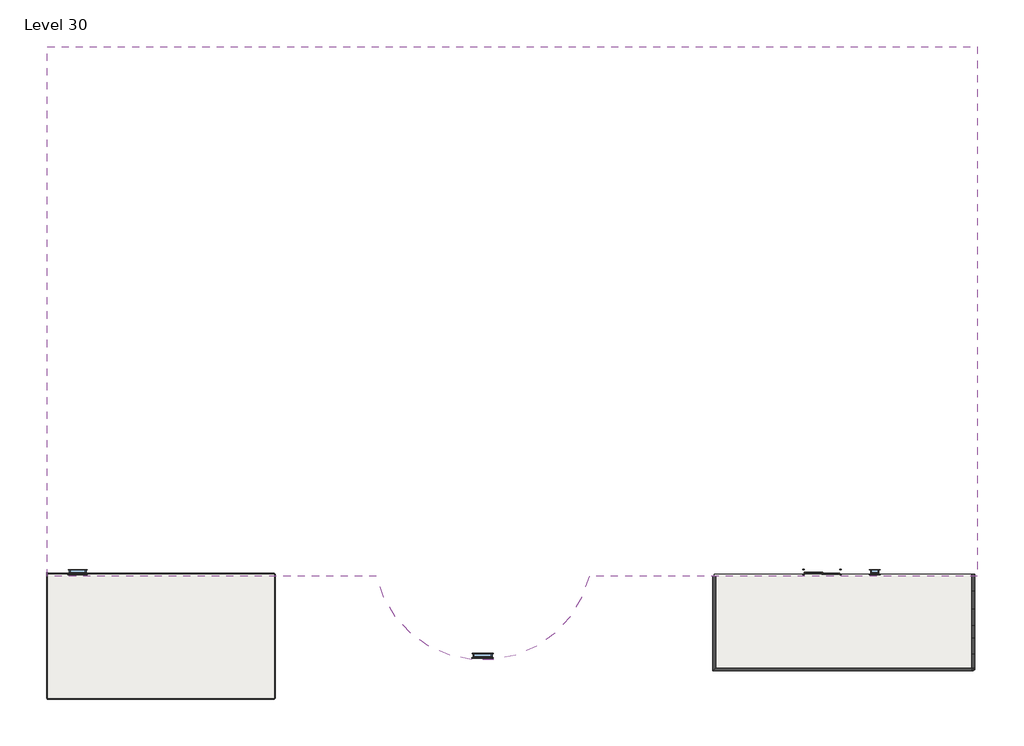
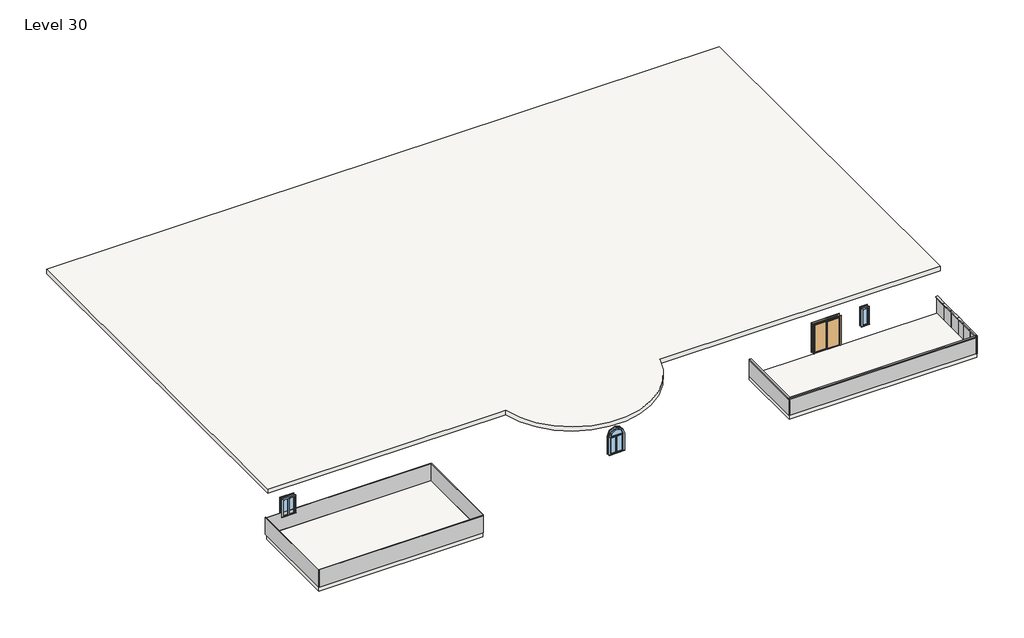
# One storey: 12 plates, 10 members, 3 slabs, 3 windows, 1 door.
"""IFC4 building model written with IfcOpenShell, lengths in millimetres."""

from ifc_helpers import new_model, si_unit, point, frame, frame_2d, origin, place, context, project, spatial, polyline, circle_curve, trimmed, segment, composite_curve, outline, extrude, transform, mapped, element, save
from components import door_076b30e0, member_75074519, member_9ef15e39, member_47bfaf8a, member_aa870034, member_b955a9e9, member_f377c62d, member_60525e8a, system_panel_glazed_689d74eb, system_panel_glazed_59c8d2f2, system_panel_glazed_7b5ce646, system_panel_glazed_f269d4c8, system_panel_glazed_7af1c9c3, system_panel_glazed_dc8eac37, system_panel_glazed_ce931456, system_panel_glazed_5fdeb3e7, system_panel_glazed_fe04ab03, window_cf4adaea, window_a765b88f, window_bb17773d

model = new_model("IFC4")

# Units and contexts
model_context = context("Model", 3, world=origin())
ifc_project = project(units=[si_unit("LENGTHUNIT", "METRE", prefix="MILLI")], contexts=[model_context])

# Site, building, storey
site = spatial("IfcSite", under=ifc_project)
building = spatial("IfcBuilding", under=site)
storey = spatial("IfcBuildingStorey", under=building, Name="Level 30", Elevation=49987.2)

# Door
placement = place(None, origin())
door_shape = door_076b30e0(model_context)
element("IfcDoor", 1, ObjectType="Door-Double-Sliding : 68\" x 80\"", at=placement, inside=storey, context=model_context, shape_type="MappedRepresentation", body=[
    mapped(door_shape, transform((17920.614721, -12227.7237084, 49987.2), x_axis=(-1.0, 0.0, 0.0), y_axis=(0.0, -1.0, 0.0), z_axis=(0.0, 0.0, 1.0))),
])

# Members
member_shape = member_75074519(model_context)
element("IfcMember", 2, ObjectType="Rectangular Mullion : 2.5\" x 5\" rectangular", at=placement, inside=storey, context=model_context, shape_type="MappedRepresentation", body=[
    mapped(member_shape, transform((25286.614721, -17112.9563074, 51206.4), x_axis=(1.0, 0.0, 0.0), y_axis=(0.0, 1.0, 0.0), z_axis=(0.0, 0.0, 1.0))),
])
member_2_shape = member_9ef15e39(model_context)
element("IfcMember", 3, ObjectType="Rectangular Mullion : 2.5\" x 5\" rectangular", at=placement, inside=storey, context=model_context, shape_type="MappedRepresentation", body=[
    mapped(member_2_shape, transform((25286.614721, -13297.3345747, 51206.4), x_axis=(0.0, 0.0, 1.0), y_axis=(-1.0, 0.0, 0.0), z_axis=(0.0, -1.0, 0.0))),
])
element("IfcMember", 4, ObjectType="Rectangular Mullion : 2.5\" x 5\" rectangular", at=placement, inside=storey, context=model_context, shape_type="MappedRepresentation", body=[
    mapped(member_2_shape, transform((25286.614721, -14138.345441, 51206.4), x_axis=(0.0, 0.0, 1.0), y_axis=(-1.0, 0.0, 0.0), z_axis=(0.0, -1.0, 0.0))),
])
element("IfcMember", 5, ObjectType="Rectangular Mullion : 2.5\" x 5\" rectangular", at=placement, inside=storey, context=model_context, shape_type="MappedRepresentation", body=[
    mapped(member_2_shape, transform((25286.614721, -14979.3563074, 51206.4), x_axis=(0.0, 0.0, 1.0), y_axis=(-1.0, 0.0, 0.0), z_axis=(0.0, -1.0, 0.0))),
])
member_3_shape = member_47bfaf8a(model_context)
element("IfcMember", 6, ObjectType="Rectangular Mullion : 2.5\" x 5\" rectangular", at=placement, inside=storey, context=model_context, shape_type="MappedRepresentation", body=[
    mapped(member_3_shape, transform((25286.614721, -15588.9563074, 51206.4), x_axis=(0.0, 0.0, 1.0), y_axis=(-1.0, 0.0, 0.0), z_axis=(0.0, -1.0, 0.0))),
])
member_4_shape = member_aa870034(model_context)
element("IfcMember", 7, ObjectType="Rectangular Mullion : 2.5\" x 5\" rectangular", at=placement, inside=storey, context=model_context, shape_type="MappedRepresentation", body=[
    mapped(member_4_shape, transform((25286.614721, -16350.9563074, 51206.4), x_axis=(0.0, 0.0, 1.0), y_axis=(-1.0, 0.0, 0.0), z_axis=(0.0, -1.0, 0.0))),
])
member_5_shape = member_b955a9e9(model_context)
element("IfcMember", 8, ObjectType="Rectangular Mullion : 2.5\" x 5\" rectangular", at=placement, inside=storey, context=model_context, shape_type="MappedRepresentation", body=[
    mapped(member_5_shape, transform((25286.614721, -17049.4563074, 51206.4), x_axis=(0.0, 0.0, 1.0), y_axis=(-1.0, 0.0, 0.0), z_axis=(0.0, -1.0, 0.0))),
])
element("IfcMember", 9, ObjectType="Rectangular Mullion : 2.5\" x 5\" rectangular", at=placement, inside=storey, context=model_context, shape_type="MappedRepresentation", body=[
    mapped(member_shape, transform((25286.614721, -17112.9563074, 49987.2), x_axis=(0.0, -1.0, 0.0), y_axis=(-1.0, 0.0, 0.0), z_axis=(0.0, 0.0, -1.0))),
])
member_6_shape = member_f377c62d(model_context)
element("IfcMember", 10, ObjectType="Rectangular Mullion : 2.5\" x 5\" rectangular", at=placement, inside=storey, context=model_context, shape_type="MappedRepresentation", body=[
    mapped(member_6_shape, transform((12667.5594464, -12557.9237084, 51206.4), x_axis=(0.0, 0.0, 1.0), y_axis=(1.0, 0.0, 0.0), z_axis=(0.0, 1.0, 0.0))),
])
member_7_shape = member_60525e8a(model_context)
element("IfcMember", 11, ObjectType="Rectangular Mullion : 2.5\" x 5\" rectangular", at=placement, inside=storey, context=model_context, shape_type="MappedRepresentation", body=[
    mapped(member_7_shape, transform((12667.5594464, -17112.9563074, 51206.4), x_axis=(0.0, 0.0, 1.0), y_axis=(0.0, 1.0, 0.0), z_axis=(-1.0, 0.0, 0.0))),
])

# Plates
system_panel_glazed_shape = system_panel_glazed_689d74eb(model_context)
element("IfcPlate", 12, ObjectType="System Panel : Glazed", at=placement, inside=storey, context=model_context, shape_type="MappedRepresentation", body=[
    mapped(system_panel_glazed_shape, transform((18945.3370837, -17112.9563074, 49987.2), x_axis=(-1.0, 0.0, 0.0), y_axis=(0.0, -1.0, 0.0), z_axis=(0.0, 0.0, 1.0))),
])
system_panel_glazed_2_shape = system_panel_glazed_59c8d2f2(model_context)
element("IfcPlate", 13, ObjectType="System Panel : Glazed", at=placement, inside=storey, context=model_context, shape_type="MappedRepresentation", body=[
    mapped(system_panel_glazed_2_shape, transform((25286.614721, -12876.8291415, 49987.2), x_axis=(0.0, -1.0, 0.0), y_axis=(1.0, 0.0, 0.0), z_axis=(0.0, 0.0, 1.0))),
])
element("IfcPlate", 14, ObjectType="System Panel : Glazed", at=placement, inside=storey, context=model_context, shape_type="MappedRepresentation", body=[
    mapped(system_panel_glazed_2_shape, transform((25286.614721, -14558.8508742, 49987.2), x_axis=(0.0, -1.0, 0.0), y_axis=(1.0, 0.0, 0.0), z_axis=(0.0, 0.0, 1.0))),
])
element("IfcPlate", 15, ObjectType="System Panel : Glazed", at=placement, inside=storey, context=model_context, shape_type="MappedRepresentation", body=[
    mapped(system_panel_glazed_2_shape, transform((25286.614721, -13717.8400079, 49987.2), x_axis=(0.0, -1.0, 0.0), y_axis=(1.0, 0.0, 0.0), z_axis=(0.0, 0.0, 1.0))),
])
system_panel_glazed_3_shape = system_panel_glazed_7b5ce646(model_context)
element("IfcPlate", 16, ObjectType="System Panel : Glazed", at=placement, inside=storey, context=model_context, shape_type="MappedRepresentation", body=[
    mapped(system_panel_glazed_3_shape, transform((25286.614721, -16700.2063074, 49987.2), x_axis=(0.0, -1.0, 0.0), y_axis=(1.0, 0.0, 0.0), z_axis=(0.0, 0.0, 1.0))),
])
system_panel_glazed_4_shape = system_panel_glazed_f269d4c8(model_context)
element("IfcPlate", 17, ObjectType="System Panel : Glazed", at=placement, inside=storey, context=model_context, shape_type="MappedRepresentation", body=[
    mapped(system_panel_glazed_4_shape, transform((25286.614721, -15969.9563074, 49987.2), x_axis=(0.0, -1.0, 0.0), y_axis=(1.0, 0.0, 0.0), z_axis=(0.0, 0.0, 1.0))),
])
system_panel_glazed_5_shape = system_panel_glazed_7af1c9c3(model_context)
element("IfcPlate", 18, ObjectType="System Panel : Glazed", at=placement, inside=storey, context=model_context, shape_type="MappedRepresentation", body=[
    mapped(system_panel_glazed_5_shape, transform((25286.614721, -15284.1563074, 49987.2), x_axis=(0.0, -1.0, 0.0), y_axis=(1.0, 0.0, 0.0), z_axis=(0.0, 0.0, 1.0))),
])
system_panel_glazed_6_shape = system_panel_glazed_dc8eac37(model_context)
element("IfcPlate", 19, ObjectType="System Panel : Glazed", at=placement, inside=storey, context=model_context, shape_type="MappedRepresentation", body=[
    mapped(system_panel_glazed_6_shape, transform((12667.5594464, -14835.4400079, 49987.2), x_axis=(0.0, 1.0, 0.0), y_axis=(-1.0, 0.0, 0.0), z_axis=(0.0, 0.0, 1.0))),
])
system_panel_glazed_7_shape = system_panel_glazed_ce931456(model_context)
element("IfcPlate", 20, ObjectType="System Panel : Glazed", at=placement, inside=storey, context=model_context, shape_type="MappedRepresentation", body=[
    mapped(system_panel_glazed_7_shape, transform((-8774.785279, -15482.0987084, 49987.2), x_axis=(0.0, -1.0, 0.0), y_axis=(1.0, 0.0, 0.0), z_axis=(0.0, 0.0, 1.0))),
])
system_panel_glazed_8_shape = system_panel_glazed_5fdeb3e7(model_context)
element("IfcPlate", 21, ObjectType="System Panel : Glazed", at=placement, inside=storey, context=model_context, shape_type="MappedRepresentation", body=[
    mapped(system_panel_glazed_8_shape, transform((-14299.285279, -12456.3237084, 49987.2), x_axis=(1.0, 0.0, 0.0), y_axis=(0.0, 1.0, 0.0), z_axis=(0.0, 0.0, 1.0))),
])
element("IfcPlate", 22, ObjectType="System Panel : Glazed", at=placement, inside=storey, context=model_context, shape_type="MappedRepresentation", body=[
    mapped(system_panel_glazed_8_shape, transform((-14299.285279, -18507.8737084, 49987.2), x_axis=(-1.0, 0.0, 0.0), y_axis=(0.0, -1.0, 0.0), z_axis=(0.0, 0.0, 1.0))),
])
system_panel_glazed_9_shape = system_panel_glazed_fe04ab03(model_context)
element("IfcPlate", 23, ObjectType="System Panel : Glazed", at=placement, inside=storey, context=model_context, shape_type="MappedRepresentation", body=[
    mapped(system_panel_glazed_9_shape, transform((-19823.785279, -15431.2987084, 49987.2), x_axis=(0.0, 1.0, 0.0), y_axis=(-1.0, 0.0, 0.0), z_axis=(0.0, 0.0, 1.0))),
])

# Slabs
element("IfcSlab", 24, ObjectType="Generic - 12\"", at=placement, inside=storey, context=model_context, shape_type="SweptSolid", body=[
    extrude(outline(composite_curve([segment(polyline([(25489.814721, 13248.6600062), (25489.814721, -12557.7399938), (6571.5594464, -12557.7399938)]), True, "CONTINUOUS"), segment(trimmed(circle_curve(frame_2d((1385.214721, -11327.1069525)), 5330.3498284), [point((6571.5594464, -12557.7399938))], [point((-3801.1300045, -12557.7399938))], False, "CARTESIAN"), True, "CONTINUOUS"), segment(polyline([(-3801.1300045, -12557.7399938), (-19823.785279, -12557.7399938), (-19823.785279, 13248.6600062), (25489.814721, 13248.6600062)]), True, "CONTINUOUS")], self_intersect=False)), frame((0.0, 0.0, 53021.7367162), z_axis=(0.0, 0.0, 1.0), x_axis=(1.0, 0.0, 0.0)), (0.0, 0.0, 1.0), 304.8),
])
element("IfcSlab", 25, ObjectType="Generic - 12\"", at=placement, inside=storey, context=model_context, shape_type="SweptSolid", body=[
    extrude(outline(polyline([(25286.614721, -12456.3237084), (25286.614721, -17112.9563074), (12667.5594464, -17112.9563074), (12667.5594464, -12456.3237084), (25286.614721, -12456.3237084)])), frame((0.0, 0.0, 49682.4), z_axis=(0.0, 0.0, 1.0), x_axis=(1.0, 0.0, 0.0)), (0.0, 0.0, 1.0), 304.8),
])
element("IfcSlab", 26, ObjectType="Generic - 12\"", at=placement, inside=storey, context=model_context, shape_type="SweptSolid", body=[
    extrude(outline(polyline([(-8781.8000285, -12456.3237084), (-8781.8000285, -18527.0702541), (-19823.785279, -18527.0702541), (-19823.785279, -12456.3237084), (-8781.8000285, -12456.3237084)])), frame((0.0, 0.0, 49682.4), z_axis=(0.0, 0.0, 1.0), x_axis=(1.0, 0.0, 0.0)), (0.0, 0.0, 1.0), 304.8),
])

# Windows
window_shape = window_cf4adaea(model_context)
element("IfcWindow", 27, ObjectType="36\" x 48\"", at=placement, inside=storey, context=model_context, shape_type="MappedRepresentation", body=[
    mapped(window_shape, transform((1388.8026463, -16434.8015058, 49987.2), x_axis=(-0.9999996409511084, 0.0008474064280801616, 0.0), y_axis=(-0.0008474064280801616, -0.9999996409511084, 0.0), z_axis=(0.0, 0.0, 1.0))),
])
window_2_shape = window_a765b88f(model_context)
element("IfcWindow", 28, ObjectType="Awning with Trim : 16\" x 48\"", at=placement, inside=storey, context=model_context, shape_type="MappedRepresentation", body=[
    mapped(window_2_shape, transform((20486.014721, -12354.7237084, 49888.7677442), x_axis=(-1.0, 0.0, 0.0), y_axis=(0.0, -1.0, 0.0), z_axis=(0.0, 0.0, 1.0))),
])
window_3_shape = window_bb17773d(model_context)
element("IfcWindow", 29, ObjectType="Casement Dbl with Trim : 32\" x 48\"", at=placement, inside=storey, context=model_context, shape_type="MappedRepresentation", body=[
    mapped(window_3_shape, transform((-18350.585279, -12335.6737084, 49987.2), x_axis=(-1.0, 0.0, 0.0), y_axis=(0.0, -1.0, 0.0), z_axis=(0.0, 0.0, 1.0))),
])

save(model, "model.ifc")

# Revit data of these elements
# Type "Door-Double-Sliding : 68\" x 80\""
#   Type Mark = "10"
#   Construction Type Id = "opn-d45"
#   Assembly Code = "C1020"
#   Analytic Construction = "Wood frame, double glass door "
#   Thickness = 0' - 2"
#   Thermal Resistance (R) = 1.8150 (h·ft²·°F)/BTU
#   Heat Transfer Coefficient (U) = 0.5510 BTU/(h·ft²·°F)
#   Height = 6' - 8"
#   Rail Width = 0' - 2"
#   Stiles = 0' - 2"
#   Trim Projection Ext = 0' - 1"
#   Trim Projection Int = 0' - 1"
#   Trim Width = 0' - 3"
#   Width = 5' - 8"
#   Define Thermal Properties by = 1
#   Glazing = Glass
#   Panel Material = Wood - Birch - Solid Stained Light Low Gloss
#   Trim Material = Paint - Sienna
#   Visual Light Transmittance = 0
#   Solar Heat Gain Coefficient = 0
#   Function = (empty or 0)
#   Wall Closure = (empty or 0)
# Type "Rectangular Mullion : 2.5\" x 5\" rectangular"
#   built-in parameter 1007304 = 0.416667 (stored number, unit not read)
#   built-in parameter 1007301 = 0.104167 (stored number, unit not read)
#   built-in parameter 1007300 = 0.104167 (stored number, unit not read)
# Type "System Panel : Glazed"
#   Construction Type Id = "GSP4R"
#   Analytic Construction = "1/8 in Pilkington single glazing"
#   Visual Light Transmittance = 0.9
#   Solar Heat Gain Coefficient = 0.86
#   Heat Transfer Coefficient (U) = 1.18115 BTU/(h·ft²·°F)
# Type "Generic - 12\""
#   Assembly Code = "B1010"
#   Function = 0
#   Layers, outside or top first: 1' - 0" no material (function 1)
# Type "36\" x 48\""
#   Type Mark = "38"
#   Construction Type Id = "SGL"
#   Assembly Code = "B2020100"
#   Analytic Construction = "Large single-glazed windows"
#   Visual Light Transmittance = 0.9
#   Solar Heat Gain Coefficient = 0.86
#   Heat Transfer Coefficient (U) = 0.979472 BTU/(h·ft²·°F)
#   Height = 4' - 0"
#   Default Sill Height = 3' - 0"
#   Trim Projection - Ext. = 0' - 0 1/2"
#   Trim Projection - Int. = 0' - 0 3/4"
#   Trim Width - Exterior = 0' - 3 1/2"
#   Trim Width - Interior = 0' - 3 1/2"
#   Width = 3' - 0"
#   Window Inset = 0' - 0 3/4"
#   Define Thermal Properties by = 1
#   Glass Pane Material = Glass
#   Sash Material = Sash
#   Trim Exterior Material = Trim
#   Trim Interior Material = Trim
#   Wall Closure = (empty or 0)
# Type "Awning with Trim : 16\" x 48\""
#   Type Mark = "14"
#   Construction Type Id = "GSP4R"
#   Assembly Code = "B2020100"
#   Analytic Construction = "1/8 in Pilkington single glazing"
#   Visual Light Transmittance = 0.9
#   Solar Heat Gain Coefficient = 0.78
#   Heat Transfer Coefficient (U) = 0.6496 BTU/(h·ft²·°F)
#   Height = 4' - 0"
#   Default Sill Height = 3' - 0"
#   Trim Projection - Ext. = 0' - 0 1/2"
#   Trim Projection - Int. = 0' - 0 3/4"
#   Trim Width - Exterior = 0' - 3 1/2"
#   Trim Width - Interior = 0' - 3 1/2"
#   Width = 1' - 4"
#   Window Inset = 0' - 0 3/4"
#   Define Thermal Properties by = 1
#   Glass Pane Material = Glass
#   Sash Material = Sash
#   Trim Exterior Material = Trim
#   Trim Interior Material = Trim
#   Wall Closure = (empty or 0)
# Type "Casement Dbl with Trim : 32\" x 48\""
#   Type Mark = "36"
#   Construction Type Id = "GSP4R"
#   Assembly Code = "B2020100"
#   Analytic Construction = "1/8 in Pilkington single glazing"
#   Visual Light Transmittance = 0.9
#   Solar Heat Gain Coefficient = 0.78
#   Heat Transfer Coefficient (U) = 0.6496 BTU/(h·ft²·°F)
#   Height = 4' - 0"
#   Default Sill Height = 3' - 0"
#   Trim Projection - Ext. = 0' - 0 1/2"
#   Trim Projection - Int. = 0' - 0 3/4"
#   Trim Width - Exterior = 0' - 3 1/2"
#   Trim Width - Interior = 0' - 3 1/2"
#   Width = 2' - 8"
#   Window Inset = 0' - 0 3/4"
#   Define Thermal Properties by = 1
#   Glass Pane Material = Glass
#   Sash Material = Sash
#   Trim Exterior Material = Trim
#   Trim Interior Material = Trim
#   Wall Closure = (empty or 0)
# Element 1 (IfcDoor, "Door-Double-Sliding : 68\" x 80\"")
#   Phase Created = New Construction
#   Materials on its faces: "Paint - Sienna", "Wood - Birch - Solid Stained Light Low Gloss", "Glass"
# Elements 2, 3, 4, 5, 6, 7, 8, 9, 10, 11 (IfcMember, "Rectangular Mullion : 2.5\" x 5\" rectangular")
#   Phase Created = New Construction
#   Materials on its faces: "Aluminum"
# Elements 12, 13, 14, 15, 16, 17, 18, 19, 20, 21, 22, 23 (IfcPlate, "System Panel : Glazed")
#   Phase Created = New Construction
#   Materials on its faces: "Glass"
# Element 24 (IfcSlab, "Generic - 12\"")
#   Height Offset From Level = 10' - 11.46995"
#   Phase Created = New Construction
#   Materials on its faces: "Default Floor"
# Elements 25, 26 (IfcSlab, "Generic - 12\"")
#   Height Offset From Level = 0' - 0"
#   Phase Created = New Construction
#   Materials on its faces: "Default Floor"
# Element 27 (IfcWindow, "36\" x 48\"")
#   Mark = "19"
#   Phase Created = New Construction
#   Materials on its faces: "Sash", "Trim", "Glass"
# Element 28 (IfcWindow, "Awning with Trim : 16\" x 48\"")
#   Mark = "53"
#   Phase Created = New Construction
#   Materials on its faces: "Sash", "Trim", "Glass"
# Element 29 (IfcWindow, "Casement Dbl with Trim : 32\" x 48\"")
#   Mark = "36"
#   Phase Created = New Construction
#   Materials on its faces: "Sash", "Trim", "Glass"
# Materials
#   "Glass": class "Glass", colour RGB 0 128 192, transparency 0.75, Description = "Soda Lime Glass", Cost = 0
#   "Wood - Birch - Solid Stained Light Low Gloss": class "Wood", colour RGB 210 159 95, transparency 0, Cost = 0
#   "Paint - Sienna": colour RGB 118 70 51, transparency 0, Cost = 0
#   "Sash": class "Wood", colour RGB 224 178 126, transparency 0
#   "Trim": class "Wood", colour RGB 224 178 126, transparency 0
#   "Aluminum": class "Metal", colour RGB 247 247 247, transparency 0, Description = "Aluminum 6061", Cost = 0
#   "Default Floor": colour RGB 128 128 128, transparency 0
